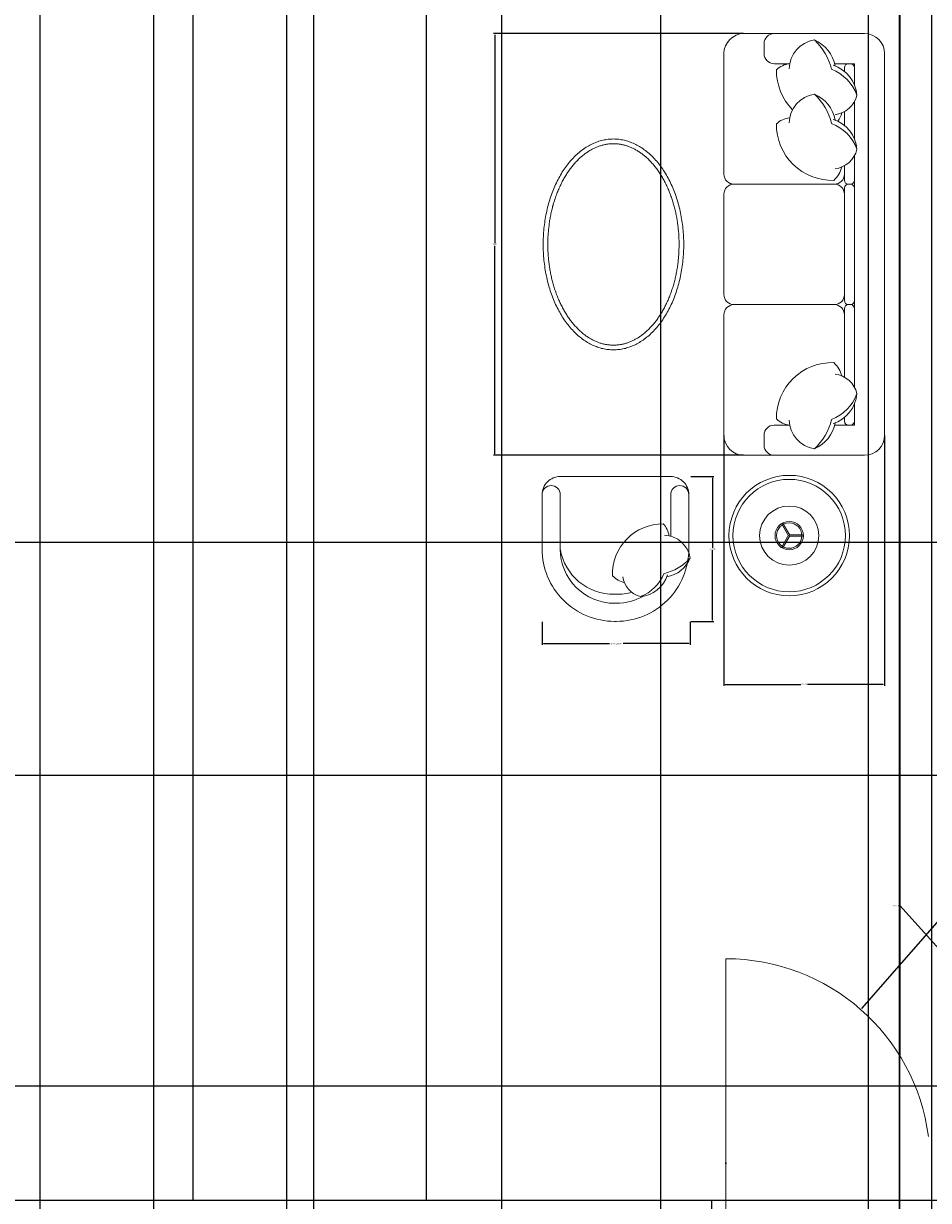
# Model space of a CAD drawing. Units: inches. Extents: x 1861 to 2564, y 1482 to 2317.
# Tile 5 of 11: x 2090 to 2217, y 1853 to 2018. Entities that reach past the tile are written whole.
import ezdxf

# ---------------------------------------------------------------- set-up
doc = ezdxf.new("R2010")
doc.units = ezdxf.units.IN
for name, color, linetype, lineweight in [('A-ANNO-DIMS', 2, 'Continuous', 18), ('A-DOOR', 3, 'Continuous', 18), ('A-FURN', 8, 'Continuous', 13), ('A-WALL', 7, 'Continuous', 35)]:
    doc.layers.add(name, color=color, linetype=linetype, lineweight=lineweight)
doc.styles.get("Standard").update_dxf_attribs({"font": 'arial.ttf'})
doc.dimstyles.get("Standard").update_dxf_attribs({"dimtxt": 0.18, "dimasz": 0.18, "dimexe": 0.18, "dimexo": 0.0625, "dimgap": 0.09, "dimtad": 0, "dimtih": 1, "dimtoh": 1, "dimdec": 4, "dimzin": 0, "dimdsep": 46, "dimtxsty": 'Standard', "dimcen": 0.09, "dimadec": 0, "dimazin": 0, "dimtfac": 1, "dimtdec": 4, "dimtofl": 0, "dimtmove": 0, "dimatfit": 3, "dimfxl": 1, "dimtolj": 1, "dimtzin": 0, "dimarcsym": 0})

# ---------------------------------------------------------------- blocks, each defined once
blk = doc.blocks.new('TABLE-SIDE-ROUND')
at = {"ltscale": 0.03}
for p, q in [((8.34, 8.45), (9.33, 10.16)), ((8.49, 8.36), (9.48, 10.08)), ((8.41, 8.5), (6.44, 8.5)), ((8.41, 8.32), (6.44, 8.32)), ((8.34, 8.36), (9.33, 6.65)), ((8.49, 8.45), (9.48, 6.74))]:
    blk.add_line(p, q, dxfattribs=at)
for radius in [8.41, 4.13, 1.98, 1.77]:
    blk.add_circle((8.41, 8.41), radius, dxfattribs=at)
blk.add_circle((8.41, 8.41), 7.85)
blk = doc.blocks.new('CHAIR-LOUNGE')
at = {"ltscale": 0.03}
blk.add_lwpolyline([(10.44, 0), (18.15, 0, 0.414214), (20.68, 2.53), (20.68, 10.11, 0.414214), (10.57, 20.22), (10.44, 20.22), (10.32, 20.22, 0.414214), (0.21, 10.11), (0.21, 2.53, 0.414214), (2.73, 0), (10.44, 0)], format="xyb", dxfattribs=at)
for points in [[(0, 11.38, -0.14773), (3.69, 13.56, -0.213343), (6.95, 16.74, -0.178662)], [(3.18, 13.73, -0.306663), (6.95, 16.74, -0.30633), (9.42, 13.99, 0.872847)], [(6.55, 16.69, -0.130591), (10.32, 17.69), (10.44, 17.69)], [(18.15, 10.11, 0.414214), (10.57, 17.69), (10.44, 17.69)], [(2.98, 8.28, 0.165541), (3.77, 6.61, 0.425989), (10.86, 13.85, 0.121523), (9.18, 14.84, -7.115464)], [(8.16, 16.16, -0.072384), (10.32, 16.43), (10.44, 16.43)], [(18.15, 10.11, 0.372719), (10.57, 16.43), (10.44, 16.43)], [(3.62, 8.2, -0.356772), (0, 11.38, -0.249542), (3.28, 14.01, 9.61688)], [(18.15, 10.11), (18.15, 2.53, 0.414214), (19.42, 1.26), (19.42, 1.26, 0.414214), (20.68, 2.53)], [(2.73, 8.34), (2.73, 2.53, -0.414214), (1.47, 1.26), (1.47, 1.26, -0.414214), (0.21, 2.53)]]:
    blk.add_lwpolyline(points, format="xyb")
blk = doc.blocks.new('TABLE-COFFEE-OVAL')
at = {"ltscale": 0.03}
blk.add_polyline3d([(9.81, 29.44, 0), (9.63, 29.44, 0), (9.44, 29.43, 0), (9.26, 29.41, 0), (9.07, 29.4, 0), (8.89, 29.37, 0), (8.7, 29.34, 0), (8.52, 29.31, 0), (8.33, 29.27, 0), (8.15, 29.23, 0), (7.97, 29.18, 0), (7.79, 29.12, 0), (7.6, 29.06, 0), (7.42, 28.99, 0), (7.24, 28.92, 0), (7.07, 28.85, 0), (6.89, 28.77, 0), (6.71, 28.68, 0), (6.54, 28.59, 0), (6.36, 28.5, 0), (6.19, 28.4, 0), (6.02, 28.29, 0), (5.85, 28.18, 0), (5.68, 28.07, 0), (5.51, 27.95, 0), (5.34, 27.82, 0), (5.18, 27.69, 0), (5.02, 27.56, 0), (4.85, 27.42, 0), (4.69, 27.28, 0), (4.54, 27.13, 0), (4.38, 26.98, 0), (4.23, 26.82, 0), (4.08, 26.66, 0), (3.93, 26.49, 0), (3.78, 26.33, 0), (3.63, 26.15, 0), (3.49, 25.97, 0), (3.35, 25.79, 0), (3.21, 25.61, 0), (3.08, 25.42, 0), (2.94, 25.23, 0), (2.81, 25.03, 0), (2.68, 24.83, 0), (2.56, 24.62, 0), (2.43, 24.42, 0), (2.31, 24.2, 0), (2.19, 23.99, 0), (2.08, 23.77, 0), (1.96, 23.55, 0), (1.85, 23.33, 0), (1.75, 23.1, 0), (1.64, 22.87, 0), (1.54, 22.63, 0), (1.44, 22.4, 0), (1.35, 22.16, 0), (1.26, 21.92, 0), (1.17, 21.67, 0), (1.08, 21.43, 0), (1, 21.18, 0), (0.92, 20.93, 0), (0.84, 20.67, 0), (0.77, 20.42, 0), (0.7, 20.16, 0), (0.63, 19.9, 0), (0.57, 19.64, 0), (0.51, 19.37, 0), (0.45, 19.11, 0), (0.39, 18.84, 0), (0.34, 18.57, 0), (0.3, 18.31, 0), (0.25, 18.03, 0), (0.21, 17.76, 0), (0.18, 17.49, 0), (0.14, 17.22, 0), (0.11, 16.94, 0), (0.09, 16.66, 0), (0.07, 16.39, 0), (0.05, 16.11, 0), (0.03, 15.83, 0), (0.02, 15.56, 0), (0.01, 15.28, 0), (0, 15, 0), (0, 14.72, 0), (0, 14.44, 0), (0.01, 14.16, 0), (0.02, 13.89, 0), (0.03, 13.61, 0), (0.05, 13.33, 0), (0.07, 13.05, 0), (0.09, 12.78, 0), (0.11, 12.5, 0), (0.14, 12.23, 0), (0.18, 11.95, 0), (0.21, 11.68, 0), (0.25, 11.41, 0), (0.3, 11.14, 0), (0.34, 10.87, 0), (0.39, 10.6, 0), (0.45, 10.33, 0), (0.51, 10.07, 0), (0.57, 9.8, 0), (0.63, 9.54, 0), (0.7, 9.28, 0), (0.77, 9.02, 0), (0.84, 8.77, 0), (0.92, 8.52, 0), (1, 8.26, 0), (1.08, 8.01, 0), (1.17, 7.77, 0), (1.26, 7.52, 0), (1.35, 7.28, 0), (1.44, 7.04, 0), (1.54, 6.81, 0), (1.64, 6.57, 0), (1.75, 6.34, 0), (1.85, 6.12, 0), (1.96, 5.89, 0), (2.08, 5.67, 0), (2.19, 5.45, 0), (2.31, 5.24, 0), (2.43, 5.03, 0), (2.56, 4.82, 0), (2.68, 4.61, 0), (2.81, 4.41, 0), (2.94, 4.22, 0), (3.08, 4.02, 0), (3.21, 3.83, 0), (3.35, 3.65, 0), (3.49, 3.47, 0), (3.63, 3.29, 0), (3.78, 3.12, 0), (3.93, 2.95, 0), (4.08, 2.78, 0), (4.23, 2.62, 0), (4.38, 2.46, 0), (4.54, 2.31, 0), (4.69, 2.17, 0), (4.85, 2.02, 0), (5.02, 1.88, 0), (5.18, 1.75, 0), (5.34, 1.62, 0), (5.51, 1.5, 0), (5.68, 1.38, 0), (5.85, 1.26, 0), (6.02, 1.15, 0), (6.19, 1.05, 0), (6.36, 0.94, 0), (6.54, 0.85, 0), (6.71, 0.76, 0), (6.89, 0.67, 0), (7.07, 0.59, 0), (7.24, 0.52, 0), (7.42, 0.45, 0), (7.6, 0.38, 0), (7.79, 0.32, 0), (7.97, 0.27, 0), (8.15, 0.22, 0), (8.33, 0.17, 0), (8.52, 0.13, 0), (8.7, 0.1, 0), (8.89, 0.07, 0), (9.07, 0.05, 0), (9.26, 0.03, 0), (9.44, 0.01, 0), (9.63, 0.01, 0), (9.81, 0, 0), (10, 0.01, 0), (10.18, 0.01, 0), (10.37, 0.03, 0), (10.56, 0.05, 0), (10.74, 0.07, 0), (10.93, 0.1, 0), (11.11, 0.13, 0), (11.29, 0.17, 0), (11.48, 0.22, 0), (11.66, 0.27, 0), (11.84, 0.32, 0), (12.02, 0.38, 0), (12.2, 0.45, 0), (12.38, 0.52, 0), (12.56, 0.59, 0), (12.74, 0.67, 0), (12.92, 0.76, 0), (13.09, 0.85, 0), (13.27, 0.94, 0), (13.44, 1.05, 0), (13.61, 1.15, 0), (13.78, 1.26, 0), (13.95, 1.38, 0), (14.12, 1.5, 0), (14.28, 1.62, 0), (14.45, 1.75, 0), (14.61, 1.88, 0), (14.77, 2.02, 0), (14.93, 2.17, 0), (15.09, 2.31, 0), (15.25, 2.46, 0), (15.4, 2.62, 0), (15.55, 2.78, 0), (15.7, 2.95, 0), (15.85, 3.12, 0), (15.99, 3.29, 0), (16.14, 3.47, 0), (16.28, 3.65, 0), (16.42, 3.83, 0), (16.55, 4.02, 0), (16.69, 4.22, 0), (16.82, 4.41, 0), (16.95, 4.61, 0), (17.07, 4.82, 0), (17.2, 5.03, 0), (17.32, 5.24, 0), (17.43, 5.45, 0), (17.55, 5.67, 0), (17.66, 5.89, 0), (17.77, 6.12, 0), (17.88, 6.34, 0), (17.98, 6.57, 0), (18.09, 6.81, 0), (18.18, 7.04, 0), (18.28, 7.28, 0), (18.37, 7.52, 0), (18.46, 7.77, 0), (18.55, 8.01, 0), (18.63, 8.26, 0), (18.71, 8.52, 0), (18.79, 8.77, 0), (18.86, 9.02, 0), (18.93, 9.28, 0), (19, 9.54, 0), (19.06, 9.8, 0), (19.12, 10.07, 0), (19.18, 10.33, 0), (19.23, 10.6, 0), (19.28, 10.87, 0), (19.33, 11.14, 0), (19.37, 11.41, 0), (19.41, 11.68, 0), (19.45, 11.95, 0), (19.48, 12.23, 0), (19.51, 12.5, 0), (19.54, 12.78, 0), (19.56, 13.05, 0), (19.58, 13.33, 0), (19.6, 13.61, 0), (19.61, 13.89, 0), (19.62, 14.16, 0), (19.62, 14.44, 0), (19.63, 14.72, 0), (19.62, 15, 0), (19.62, 15.28, 0), (19.61, 15.56, 0), (19.6, 15.83, 0), (19.58, 16.11, 0), (19.56, 16.39, 0), (19.54, 16.66, 0), (19.51, 16.94, 0), (19.48, 17.22, 0), (19.45, 17.49, 0), (19.41, 17.76, 0), (19.37, 18.03, 0), (19.33, 18.31, 0), (19.28, 18.57, 0), (19.23, 18.84, 0), (19.18, 19.11, 0), (19.12, 19.37, 0), (19.06, 19.64, 0), (19, 19.9, 0), (18.93, 20.16, 0), (18.86, 20.42, 0), (18.79, 20.67, 0), (18.71, 20.93, 0), (18.63, 21.18, 0), (18.55, 21.43, 0), (18.46, 21.67, 0), (18.37, 21.92, 0), (18.28, 22.16, 0), (18.18, 22.4, 0), (18.09, 22.63, 0), (17.98, 22.87, 0), (17.88, 23.1, 0), (17.77, 23.33, 0), (17.66, 23.55, 0), (17.55, 23.77, 0), (17.43, 23.99, 0), (17.32, 24.2, 0), (17.2, 24.42, 0), (17.07, 24.62, 0), (16.95, 24.83, 0), (16.82, 25.03, 0), (16.69, 25.23, 0), (16.55, 25.42, 0), (16.42, 25.61, 0), (16.28, 25.79, 0), (16.14, 25.97, 0), (15.99, 26.15, 0), (15.85, 26.33, 0), (15.7, 26.49, 0), (15.55, 26.66, 0), (15.4, 26.82, 0), (15.25, 26.98, 0), (15.09, 27.13, 0), (14.93, 27.28, 0), (14.77, 27.42, 0), (14.61, 27.56, 0), (14.45, 27.69, 0), (14.28, 27.82, 0), (14.12, 27.95, 0), (13.95, 28.07, 0), (13.78, 28.18, 0), (13.61, 28.29, 0), (13.44, 28.4, 0), (13.27, 28.5, 0), (13.09, 28.59, 0), (12.92, 28.68, 0), (12.74, 28.77, 0), (12.56, 28.85, 0), (12.38, 28.92, 0), (12.2, 28.99, 0), (12.02, 29.06, 0), (11.84, 29.12, 0), (11.66, 29.18, 0), (11.48, 29.23, 0), (11.29, 29.27, 0), (11.11, 29.31, 0), (10.93, 29.34, 0), (10.74, 29.37, 0), (10.56, 29.4, 0), (10.37, 29.41, 0), (10.18, 29.43, 0), (10, 29.44, 0), (9.81, 29.44, 0)], dxfattribs=at)
blk.add_polyline3d([(9.81, 28.78, 0), (9.71, 28.78, 0), (9.61, 28.78, 0), (9.51, 28.78, 0), (9.41, 28.77, 0), (9.31, 28.76, 0), (9.2, 28.75, 0), (9.1, 28.74, 0), (9, 28.73, 0), (8.89, 28.71, 0), (8.79, 28.69, 0), (8.69, 28.68, 0), (8.58, 28.65, 0), (8.48, 28.63, 0), (8.37, 28.61, 0), (8.27, 28.58, 0), (8.16, 28.55, 0), (8.05, 28.52, 0), (7.95, 28.49, 0), (7.84, 28.45, 0), (7.73, 28.41, 0), (7.63, 28.37, 0), (7.52, 28.33, 0), (7.41, 28.29, 0), (7.31, 28.24, 0), (7.2, 28.19, 0), (7.09, 28.14, 0), (6.98, 28.09, 0), (6.88, 28.03, 0), (6.77, 27.97, 0), (6.66, 27.91, 0), (6.55, 27.85, 0), (6.45, 27.79, 0), (6.34, 27.72, 0), (6.23, 27.65, 0), (6.13, 27.58, 0), (6.02, 27.51, 0), (5.92, 27.43, 0), (5.81, 27.36, 0), (5.71, 27.28, 0), (5.6, 27.19, 0), (5.5, 27.11, 0), (5.39, 27.02, 0), (5.29, 26.93, 0), (5.19, 26.84, 0), (5.09, 26.75, 0), (4.98, 26.65, 0), (4.88, 26.55, 0), (4.78, 26.45, 0), (4.68, 26.34, 0), (4.58, 26.24, 0), (4.49, 26.13, 0), (4.39, 26.02, 0), (4.29, 25.91, 0), (4.2, 25.79, 0), (4.1, 25.68, 0), (4.01, 25.56, 0), (3.91, 25.44, 0), (3.82, 25.32, 0), (3.73, 25.19, 0), (3.64, 25.07, 0), (3.55, 24.94, 0), (3.46, 24.81, 0), (3.37, 24.68, 0), (3.29, 24.54, 0), (3.2, 24.41, 0), (3.12, 24.27, 0), (3.03, 24.13, 0), (2.95, 23.99, 0), (2.87, 23.85, 0), (2.79, 23.71, 0), (2.71, 23.56, 0), (2.63, 23.41, 0), (2.56, 23.27, 0), (2.48, 23.12, 0), (2.41, 22.97, 0), (2.34, 22.81, 0), (2.27, 22.66, 0), (2.2, 22.51, 0), (2.13, 22.35, 0), (2.07, 22.19, 0), (2, 22.04, 0), (1.94, 21.88, 0), (1.88, 21.72, 0), (1.82, 21.55, 0), (1.76, 21.39, 0), (1.7, 21.23, 0), (1.65, 21.07, 0), (1.6, 20.9, 0), (1.54, 20.74, 0), (1.49, 20.58, 0), (1.44, 20.41, 0), (1.4, 20.25, 0), (1.35, 20.08, 0), (1.31, 19.92, 0), (1.26, 19.75, 0), (1.22, 19.59, 0), (1.18, 19.42, 0), (1.15, 19.25, 0), (1.11, 19.09, 0), (1.07, 18.92, 0), (1.04, 18.75, 0), (1.01, 18.58, 0), (0.98, 18.42, 0), (0.95, 18.25, 0), (0.92, 18.08, 0), (0.89, 17.91, 0), (0.87, 17.74, 0), (0.84, 17.57, 0), (0.82, 17.4, 0), (0.8, 17.23, 0), (0.78, 17.06, 0), (0.76, 16.89, 0), (0.75, 16.72, 0), (0.73, 16.55, 0), (0.72, 16.38, 0), (0.71, 16.21, 0), (0.7, 16.04, 0), (0.69, 15.87, 0), (0.68, 15.7, 0), (0.67, 15.53, 0), (0.67, 15.36, 0), (0.66, 15.19, 0), (0.66, 15.02, 0), (0.66, 14.85, 0), (0.66, 14.68, 0), (0.66, 14.51, 0), (0.66, 14.34, 0), (0.66, 14.17, 0), (0.67, 14, 0), (0.67, 13.82, 0), (0.68, 13.65, 0), (0.69, 13.48, 0), (0.7, 13.31, 0), (0.71, 13.14, 0), (0.73, 12.97, 0), (0.74, 12.8, 0), (0.76, 12.63, 0), (0.77, 12.46, 0), (0.79, 12.29, 0), (0.81, 12.12, 0), (0.83, 11.95, 0), (0.86, 11.78, 0), (0.88, 11.62, 0), (0.91, 11.45, 0), (0.93, 11.28, 0), (0.96, 11.11, 0), (0.99, 10.94, 0), (1.02, 10.77, 0), (1.06, 10.61, 0), (1.09, 10.44, 0), (1.13, 10.27, 0), (1.16, 10.1, 0), (1.2, 9.94, 0), (1.24, 9.77, 0), (1.29, 9.61, 0), (1.33, 9.44, 0), (1.37, 9.28, 0), (1.42, 9.11, 0), (1.47, 8.95, 0), (1.52, 8.78, 0), (1.57, 8.62, 0), (1.62, 8.46, 0), (1.68, 8.29, 0), (1.73, 8.13, 0), (1.79, 7.97, 0), (1.85, 7.81, 0), (1.91, 7.65, 0), (1.97, 7.49, 0), (2.03, 7.33, 0), (2.1, 7.17, 0), (2.17, 7.01, 0), (2.23, 6.86, 0), (2.3, 6.7, 0), (2.37, 6.55, 0), (2.45, 6.4, 0), (2.52, 6.25, 0), (2.6, 6.1, 0), (2.67, 5.95, 0), (2.75, 5.81, 0), (2.83, 5.66, 0), (2.91, 5.52, 0), (2.99, 5.38, 0), (3.07, 5.24, 0), (3.16, 5.1, 0), (3.24, 4.97, 0), (3.33, 4.83, 0), (3.42, 4.7, 0), (3.5, 4.57, 0), (3.59, 4.44, 0), (3.68, 4.31, 0), (3.77, 4.19, 0), (3.87, 4.06, 0), (3.96, 3.94, 0), (4.05, 3.82, 0), (4.15, 3.71, 0), (4.24, 3.59, 0), (4.34, 3.48, 0), (4.44, 3.37, 0), (4.53, 3.26, 0), (4.63, 3.15, 0), (4.73, 3.04, 0), (4.83, 2.94, 0), (4.93, 2.84, 0), (5.03, 2.74, 0), (5.14, 2.65, 0), (5.24, 2.56, 0), (5.34, 2.47, 0), (5.44, 2.38, 0), (5.55, 2.29, 0), (5.65, 2.21, 0), (5.76, 2.13, 0), (5.86, 2.05, 0), (5.97, 1.97, 0), (6.07, 1.9, 0), (6.18, 1.82, 0), (6.29, 1.75, 0), (6.39, 1.69, 0), (6.5, 1.62, 0), (6.61, 1.56, 0), (6.72, 1.5, 0), (6.82, 1.44, 0), (6.93, 1.38, 0), (7.04, 1.33, 0), (7.14, 1.28, 0), (7.25, 1.23, 0), (7.36, 1.18, 0), (7.47, 1.13, 0), (7.57, 1.09, 0), (7.68, 1.05, 0), (7.79, 1.01, 0), (7.89, 0.97, 0), (8, 0.94, 0), (8.11, 0.91, 0), (8.21, 0.88, 0), (8.32, 0.85, 0), (8.42, 0.82, 0), (8.53, 0.8, 0), (8.63, 0.78, 0), (8.74, 0.76, 0), (8.84, 0.74, 0), (8.95, 0.72, 0), (9.05, 0.71, 0), (9.15, 0.69, 0), (9.26, 0.68, 0), (9.36, 0.68, 0), (9.46, 0.67, 0), (9.56, 0.66, 0), (9.66, 0.66, 0), (9.76, 0.66, 0), (9.86, 0.66, 0), (9.96, 0.66, 0), (10.07, 0.66, 0), (10.17, 0.67, 0), (10.27, 0.68, 0), (10.37, 0.68, 0), (10.47, 0.69, 0), (10.58, 0.71, 0), (10.68, 0.72, 0), (10.78, 0.74, 0), (10.89, 0.76, 0), (10.99, 0.78, 0), (11.1, 0.8, 0), (11.2, 0.82, 0), (11.31, 0.85, 0), (11.41, 0.88, 0), (11.52, 0.91, 0), (11.63, 0.94, 0), (11.73, 0.97, 0), (11.84, 1.01, 0), (11.95, 1.05, 0), (12.05, 1.09, 0), (12.16, 1.13, 0), (12.27, 1.18, 0), (12.37, 1.23, 0), (12.48, 1.28, 0), (12.59, 1.33, 0), (12.7, 1.38, 0), (12.8, 1.44, 0), (12.91, 1.5, 0), (13.02, 1.56, 0), (13.13, 1.62, 0), (13.23, 1.69, 0), (13.34, 1.75, 0), (13.45, 1.82, 0), (13.55, 1.9, 0), (13.66, 1.97, 0), (13.76, 2.05, 0), (13.87, 2.13, 0), (13.97, 2.21, 0), (14.08, 2.29, 0), (14.18, 2.38, 0), (14.29, 2.47, 0), (14.39, 2.56, 0), (14.49, 2.65, 0), (14.59, 2.74, 0), (14.69, 2.84, 0), (14.79, 2.94, 0), (14.89, 3.04, 0), (14.99, 3.15, 0), (15.09, 3.26, 0), (15.19, 3.37, 0), (15.29, 3.48, 0), (15.38, 3.59, 0), (15.48, 3.71, 0), (15.57, 3.82, 0), (15.67, 3.94, 0), (15.76, 4.06, 0), (15.85, 4.19, 0), (15.94, 4.31, 0), (16.03, 4.44, 0), (16.12, 4.57, 0), (16.21, 4.7, 0), (16.3, 4.83, 0), (16.38, 4.97, 0), (16.47, 5.1, 0), (16.55, 5.24, 0), (16.64, 5.38, 0), (16.72, 5.52, 0), (16.8, 5.66, 0), (16.88, 5.81, 0), (16.95, 5.95, 0), (17.03, 6.1, 0), (17.11, 6.25, 0), (17.18, 6.4, 0), (17.25, 6.55, 0), (17.32, 6.7, 0), (17.39, 6.86, 0), (17.46, 7.01, 0), (17.53, 7.17, 0), (17.59, 7.33, 0), (17.66, 7.49, 0), (17.72, 7.65, 0), (17.78, 7.81, 0), (17.84, 7.97, 0), (17.9, 8.13, 0), (17.95, 8.29, 0), (18.01, 8.46, 0), (18.06, 8.62, 0), (18.11, 8.78, 0), (18.16, 8.95, 0), (18.21, 9.11, 0), (18.25, 9.28, 0), (18.3, 9.44, 0), (18.34, 9.61, 0), (18.38, 9.77, 0), (18.42, 9.94, 0), (18.46, 10.1, 0), (18.5, 10.27, 0), (18.54, 10.44, 0), (18.57, 10.61, 0), (18.6, 10.77, 0), (18.63, 10.94, 0), (18.66, 11.11, 0), (18.69, 11.28, 0), (18.72, 11.45, 0), (18.75, 11.62, 0), (18.77, 11.78, 0), (18.79, 11.95, 0), (18.81, 12.12, 0), (18.83, 12.29, 0), (18.85, 12.46, 0), (18.87, 12.63, 0), (18.89, 12.8, 0), (18.9, 12.97, 0), (18.91, 13.14, 0), (18.93, 13.31, 0), (18.94, 13.48, 0), (18.95, 13.65, 0), (18.95, 13.82, 0), (18.96, 14, 0), (18.96, 14.17, 0), (18.97, 14.34, 0), (18.97, 14.51, 0), (18.97, 14.68, 0), (18.97, 14.85, 0), (18.97, 15.02, 0), (18.97, 15.19, 0), (18.96, 15.36, 0), (18.96, 15.53, 0), (18.95, 15.7, 0), (18.94, 15.87, 0), (18.93, 16.04, 0), (18.92, 16.21, 0), (18.91, 16.38, 0), (18.89, 16.55, 0), (18.88, 16.72, 0), (18.86, 16.89, 0), (18.84, 17.06, 0), (18.83, 17.23, 0), (18.8, 17.4, 0), (18.78, 17.57, 0), (18.76, 17.74, 0), (18.73, 17.91, 0), (18.71, 18.08, 0), (18.68, 18.25, 0), (18.65, 18.42, 0), (18.62, 18.58, 0), (18.59, 18.75, 0), (18.55, 18.92, 0), (18.52, 19.09, 0), (18.48, 19.25, 0), (18.44, 19.42, 0), (18.4, 19.59, 0), (18.36, 19.75, 0), (18.32, 19.92, 0), (18.28, 20.08, 0), (18.23, 20.25, 0), (18.18, 20.41, 0), (18.13, 20.58, 0), (18.08, 20.74, 0), (18.03, 20.9, 0), (17.98, 21.07, 0), (17.92, 21.23, 0), (17.87, 21.39, 0), (17.81, 21.55, 0), (17.75, 21.72, 0), (17.69, 21.88, 0), (17.62, 22.04, 0), (17.56, 22.19, 0), (17.49, 22.35, 0), (17.43, 22.51, 0), (17.36, 22.66, 0), (17.29, 22.81, 0), (17.22, 22.97, 0), (17.14, 23.12, 0), (17.07, 23.27, 0), (16.99, 23.41, 0), (16.92, 23.56, 0), (16.84, 23.71, 0), (16.76, 23.85, 0), (16.68, 23.99, 0), (16.59, 24.13, 0), (16.51, 24.27, 0), (16.43, 24.41, 0), (16.34, 24.54, 0), (16.26, 24.68, 0), (16.17, 24.81, 0), (16.08, 24.94, 0), (15.99, 25.07, 0), (15.9, 25.19, 0), (15.81, 25.32, 0), (15.71, 25.44, 0), (15.62, 25.56, 0), (15.53, 25.68, 0), (15.43, 25.79, 0), (15.34, 25.91, 0), (15.24, 26.02, 0), (15.14, 26.13, 0), (15.04, 26.24, 0), (14.94, 26.34, 0), (14.84, 26.45, 0), (14.74, 26.55, 0), (14.64, 26.65, 0), (14.54, 26.75, 0), (14.44, 26.84, 0), (14.34, 26.93, 0), (14.23, 27.02, 0), (14.13, 27.11, 0), (14.03, 27.19, 0), (13.92, 27.28, 0), (13.82, 27.36, 0), (13.71, 27.43, 0), (13.61, 27.51, 0), (13.5, 27.58, 0), (13.39, 27.65, 0), (13.29, 27.72, 0), (13.18, 27.79, 0), (13.07, 27.85, 0), (12.97, 27.91, 0), (12.86, 27.97, 0), (12.75, 28.03, 0), (12.64, 28.09, 0), (12.54, 28.14, 0), (12.43, 28.19, 0), (12.32, 28.24, 0), (12.21, 28.29, 0), (12.11, 28.33, 0), (12, 28.37, 0), (11.89, 28.41, 0), (11.79, 28.45, 0), (11.68, 28.49, 0), (11.57, 28.52, 0), (11.47, 28.55, 0), (11.36, 28.58, 0), (11.26, 28.61, 0), (11.15, 28.63, 0), (11.05, 28.65, 0), (10.94, 28.68, 0), (10.84, 28.69, 0), (10.73, 28.71, 0), (10.63, 28.73, 0), (10.53, 28.74, 0), (10.42, 28.75, 0), (10.32, 28.76, 0), (10.22, 28.77, 0), (10.12, 28.78, 0), (10.01, 28.78, 0), (9.91, 28.78, 0), (9.81, 28.78, 0)])
blk = doc.blocks.new('*D26')
at = {"layer": 'A-ANNO-DIMS', "color": 0, "lineweight": -2, "transparency": 16777216}
for p, q in [((2162.87, 1934.17), (2162.87, 1930.95)), ((2183.55, 1934.17), (2183.55, 1930.95)), ((2163.05, 1931.13), (2172.26, 1931.13)), ((2183.37, 1931.13), (2174.17, 1931.13))]:
    blk.add_line(p, q, dxfattribs=at)
at = {"layer": 'A-ANNO-DIMS', "color": 0, "transparency": 16777216}
for points in [[(2163.05, 1931.16), (2163.05, 1931.1), (2162.87, 1931.13)], [(2183.37, 1931.16), (2183.37, 1931.1), (2183.55, 1931.13)]]:
    blk.add_solid(points, dxfattribs=at)
at = {"layer": 'Defpoints', "color": 0, "transparency": 16777216}
for p in [(2162.87, 1934.23), (2183.55, 1934.23), (2162.87, 1931.13)]:
    blk.add_point(p, dxfattribs=at)
at = {"layer": 'A-ANNO-DIMS', "color": 0, "transparency": 16777216, "insert": (2173.21, 1931.13), "char_height": 0.18, "attachment_point": 5}
blk.add_mtext('\\A1;CHAIR 21 TYP.', dxfattribs=at)
blk = doc.blocks.new('*D27')
at = {"layer": 'A-ANNO-DIMS', "color": 0, "lineweight": -2, "transparency": 16777216}
for p, q in [((2183.62, 1954.45), (2186.84, 1954.45)), ((2186.66, 1954.27), (2186.66, 1944.52)), ((2186.66, 1934.41), (2186.66, 1944.16)), ((2183.62, 1934.23), (2186.84, 1934.23))]:
    blk.add_line(p, q, dxfattribs=at)
at = {"layer": 'A-ANNO-DIMS', "color": 0, "transparency": 16777216}
for points in [[(2186.63, 1954.27), (2186.69, 1954.27), (2186.66, 1954.45)], [(2186.63, 1934.41), (2186.69, 1934.41), (2186.66, 1934.23)]]:
    blk.add_solid(points, dxfattribs=at)
at = {"layer": 'Defpoints', "color": 0, "transparency": 16777216}
for p in [(2183.55, 1954.45), (2183.55, 1934.23), (2186.66, 1934.23)]:
    blk.add_point(p, dxfattribs=at)
at = {"layer": 'A-ANNO-DIMS', "color": 0, "transparency": 16777216, "insert": (2186.66, 1944.34), "char_height": 0.18, "attachment_point": 5}
blk.add_mtext('\\A1;20 TYP.', dxfattribs=at)
blk = doc.blocks.new('*D36')
at = {"layer": 'A-ANNO-DIMS', "color": 0, "lineweight": -2, "transparency": 16777216}
for p, q in [((2092.74, 2250.82), (2092.74, 1545.6)), ((2127.18, 2250.82), (2127.18, 1545.6)), ((2092.92, 1545.78), (2109.5, 1545.78)), ((2127, 1545.78), (2110.43, 1545.78))]:
    blk.add_line(p, q, dxfattribs=at)
at = {"layer": 'A-ANNO-DIMS', "color": 0, "transparency": 16777216}
for points in [[(2092.92, 1545.81), (2092.92, 1545.75), (2092.74, 1545.78)], [(2127, 1545.81), (2127, 1545.75), (2127.18, 1545.78)]]:
    blk.add_solid(points, dxfattribs=at)
at = {"layer": 'Defpoints', "color": 0, "transparency": 16777216}
for p in [(2092.74, 2250.89), (2127.18, 2250.89), (2127.18, 1545.78)]:
    blk.add_point(p, dxfattribs=at)
at = {"layer": 'A-ANNO-DIMS', "color": 0, "transparency": 16777216, "insert": (2109.96, 1545.78), "char_height": 0.18, "attachment_point": 5}
blk.add_mtext('\\A1;34.445', dxfattribs=at)
blk = doc.blocks.new('*D52')
at = {"layer": 'A-ANNO-DIMS', "color": 0, "lineweight": -2, "transparency": 16777216}
for p, q in [((2179.39, 2154.82), (2179.39, 1545.6)), ((2208.37, 2154.82), (2208.37, 1545.6)), ((2179.57, 1545.78), (2193.49, 1545.78)), ((2208.19, 1545.78), (2194.28, 1545.78))]:
    blk.add_line(p, q, dxfattribs=at)
at = {"layer": 'A-ANNO-DIMS', "color": 0, "transparency": 16777216}
for points in [[(2179.57, 1545.81), (2179.57, 1545.75), (2179.39, 1545.78)], [(2208.19, 1545.81), (2208.19, 1545.75), (2208.37, 1545.78)]]:
    blk.add_solid(points, dxfattribs=at)
at = {"layer": 'Defpoints', "color": 0, "transparency": 16777216}
for p in [(2179.39, 2154.89), (2208.37, 2154.89), (2208.37, 1545.78)]:
    blk.add_point(p, dxfattribs=at)
at = {"layer": 'A-ANNO-DIMS', "color": 0, "transparency": 16777216, "insert": (2193.88, 1545.78), "char_height": 0.18, "attachment_point": 5}
blk.add_mtext('\\A1;28.98', dxfattribs=at)
blk = doc.blocks.new('*D53')
at = {"layer": 'A-ANNO-DIMS', "color": 0, "lineweight": -2, "transparency": 16777216}
for p, q in [((2076.3, 1945.29), (2537.22, 1945.29)), ((2537.04, 1945.11), (2537.04, 1929.2)), ((2537.04, 1912.93), (2537.04, 1928.84)), ((2076.3, 1912.75), (2537.22, 1912.75))]:
    blk.add_line(p, q, dxfattribs=at)
at = {"layer": 'A-ANNO-DIMS', "color": 0, "transparency": 16777216}
for points in [[(2537.01, 1945.11), (2537.07, 1945.11), (2537.04, 1945.29)], [(2537.01, 1912.93), (2537.07, 1912.93), (2537.04, 1912.75)]]:
    blk.add_solid(points, dxfattribs=at)
at = {"layer": 'Defpoints', "color": 0, "transparency": 16777216}
for p in [(2076.24, 1945.29), (2537.04, 1945.29), (2076.24, 1912.75)]:
    blk.add_point(p, dxfattribs=at)
at = {"layer": 'A-ANNO-DIMS', "color": 0, "transparency": 16777216, "insert": (2537.04, 1929.02), "char_height": 0.18, "attachment_point": 5}
blk.add_mtext('\\A1;32.544', dxfattribs=at)
blk = doc.blocks.new('*D55')
at = {"layer": 'A-ANNO-DIMS', "color": 0, "lineweight": -2, "transparency": 16777216}
for p, q in [((2114.18, 1853.45), (2114.18, 2290.37)), ((2114.36, 2290.19), (2130, 2290.19)), ((2146.56, 2290.19), (2130.92, 2290.19)), ((2146.74, 1853.45), (2146.74, 2290.37))]:
    blk.add_line(p, q, dxfattribs=at)
at = {"layer": 'A-ANNO-DIMS', "color": 0, "transparency": 16777216}
for points in [[(2114.36, 2290.22), (2114.36, 2290.16), (2114.18, 2290.19)], [(2146.56, 2290.22), (2146.56, 2290.16), (2146.74, 2290.19)]]:
    blk.add_solid(points, dxfattribs=at)
at = {"layer": 'Defpoints', "color": 0, "transparency": 16777216}
for p in [(2146.74, 2290.19), (2114.18, 1853.39), (2146.74, 1853.39)]:
    blk.add_point(p, dxfattribs=at)
at = {"layer": 'A-ANNO-DIMS', "color": 0, "transparency": 16777216, "insert": (2130.46, 2290.19), "char_height": 0.18, "attachment_point": 5}
blk.add_mtext('\\A1;32.564', dxfattribs=at)
blk = doc.blocks.new('*D56')
at = {"layer": 'A-ANNO-DIMS', "color": 0, "lineweight": -2, "transparency": 16777216}
for p, q in [((2186.51, 1853.32), (2186.51, 1545.6)), ((2244.44, 1853.32), (2244.44, 1545.6)), ((2186.69, 1545.78), (2215.08, 1545.78)), ((2244.26, 1545.78), (2215.87, 1545.78))]:
    blk.add_line(p, q, dxfattribs=at)
at = {"layer": 'A-ANNO-DIMS', "color": 0, "transparency": 16777216}
for points in [[(2186.69, 1545.81), (2186.69, 1545.75), (2186.51, 1545.78)], [(2244.26, 1545.81), (2244.26, 1545.75), (2244.44, 1545.78)]]:
    blk.add_solid(points, dxfattribs=at)
at = {"layer": 'Defpoints', "color": 0, "transparency": 16777216}
for p in [(2186.51, 1853.39), (2244.44, 1853.39), (2244.44, 1545.78)]:
    blk.add_point(p, dxfattribs=at)
at = {"layer": 'A-ANNO-DIMS', "color": 0, "transparency": 16777216, "insert": (2215.48, 1545.78), "char_height": 0.18, "attachment_point": 5}
blk.add_mtext('\\A1;57.93', dxfattribs=at)
blk = doc.blocks.new('*D58')
at = {"layer": 'A-ANNO-DIMS', "color": 0, "lineweight": -2, "transparency": 16777216}
for p, q in [((2190.99, 2016.29), (2156.07, 2016.29)), ((2156.25, 2016.11), (2156.25, 1987.04)), ((2156.25, 1957.6), (2156.25, 1986.67)), ((2190.99, 1957.42), (2156.07, 1957.42))]:
    blk.add_line(p, q, dxfattribs=at)
at = {"layer": 'A-ANNO-DIMS', "color": 0, "transparency": 16777216}
for points in [[(2156.22, 2016.11), (2156.28, 2016.11), (2156.25, 2016.29)], [(2156.22, 1957.6), (2156.28, 1957.6), (2156.25, 1957.42)]]:
    blk.add_solid(points, dxfattribs=at)
at = {"layer": 'Defpoints', "color": 0, "transparency": 16777216}
for p in [(2156.25, 2016.29), (2191.05, 2016.29), (2191.05, 1957.42)]:
    blk.add_point(p, dxfattribs=at)
at = {"layer": 'A-ANNO-DIMS', "color": 0, "transparency": 16777216, "insert": (2156.25, 1986.86), "char_height": 0.18, "attachment_point": 5}
blk.add_mtext('\\A1;58.87', dxfattribs=at)
blk = doc.blocks.new('*D59')
at = {"layer": 'A-ANNO-DIMS', "color": 0, "lineweight": -2, "transparency": 16777216}
for p, q in [((2188.25, 1960.16), (2188.25, 1925.25)), ((2210.67, 1960.16), (2210.67, 1925.25)), ((2188.43, 1925.43), (2199, 1925.43)), ((2210.49, 1925.43), (2199.93, 1925.43))]:
    blk.add_line(p, q, dxfattribs=at)
at = {"layer": 'A-ANNO-DIMS', "color": 0, "transparency": 16777216}
for points in [[(2188.43, 1925.46), (2188.43, 1925.4), (2188.25, 1925.43)], [(2210.49, 1925.46), (2210.49, 1925.4), (2210.67, 1925.43)]]:
    blk.add_solid(points, dxfattribs=at)
at = {"layer": 'Defpoints', "color": 0, "transparency": 16777216}
for p in [(2188.25, 1960.23), (2210.67, 1960.23), (2188.25, 1925.43)]:
    blk.add_point(p, dxfattribs=at)
at = {"layer": 'A-ANNO-DIMS', "color": 0, "transparency": 16777216, "insert": (2199.46, 1925.43), "char_height": 0.18, "attachment_point": 5}
blk.add_mtext('\\A1;22.426', dxfattribs=at)
blk = doc.blocks.new('*D62')
at = {"layer": 'A-ANNO-DIMS', "color": 0, "lineweight": -2, "transparency": 16777216}
for p, q in [((2108.68, 1781.45), (2108.68, 2290.37)), ((2108.86, 2290.19), (2119.46, 2290.19)), ((2130.84, 2290.19), (2120.25, 2290.19)), ((2131.02, 1781.45), (2131.02, 2290.37))]:
    blk.add_line(p, q, dxfattribs=at)
at = {"layer": 'A-ANNO-DIMS', "color": 0, "transparency": 16777216}
for points in [[(2108.86, 2290.22), (2108.86, 2290.16), (2108.68, 2290.19)], [(2130.84, 2290.22), (2130.84, 2290.16), (2131.02, 2290.19)]]:
    blk.add_solid(points, dxfattribs=at)
at = {"layer": 'Defpoints', "color": 0, "transparency": 16777216}
for p in [(2131.02, 2290.19), (2108.68, 1781.39), (2131.02, 1781.39)]:
    blk.add_point(p, dxfattribs=at)
at = {"layer": 'A-ANNO-DIMS', "color": 0, "transparency": 16777216, "insert": (2119.85, 2290.19), "char_height": 0.18, "attachment_point": 5}
blk.add_mtext('\\A1;22.34', dxfattribs=at)
blk = doc.blocks.new('*D66')
at = {"layer": 'A-ANNO-DIMS', "color": 0, "lineweight": -2, "transparency": 16777216}
for p, q in [((2497.68, 1869.33), (1892.76, 1869.33)), ((1892.94, 1869.15), (1892.94, 1861.54)), ((1892.94, 1853.57), (1892.94, 1861.17)), ((2497.68, 1853.39), (1892.76, 1853.39))]:
    blk.add_line(p, q, dxfattribs=at)
at = {"layer": 'A-ANNO-DIMS', "color": 0, "transparency": 16777216}
for points in [[(1892.91, 1869.15), (1892.97, 1869.15), (1892.94, 1869.33)], [(1892.91, 1853.57), (1892.97, 1853.57), (1892.94, 1853.39)]]:
    blk.add_solid(points, dxfattribs=at)
at = {"layer": 'Defpoints', "color": 0, "transparency": 16777216}
for p in [(2497.74, 1869.33), (1892.94, 1853.39), (2497.74, 1853.39)]:
    blk.add_point(p, dxfattribs=at)
at = {"layer": 'A-ANNO-DIMS', "color": 0, "transparency": 16777216, "insert": (1892.94, 1861.36), "char_height": 0.18, "attachment_point": 5}
blk.add_mtext('\\A1;15.94', dxfattribs=at)
blk = doc.blocks.new('*D68')
at = {"layer": 'A-ANNO-DIMS', "color": 0, "lineweight": -2, "transparency": 16777216}
for p, q in [((2157.24, 1794.95), (2157.24, 2290.37)), ((2157.42, 2290.19), (2184.66, 2290.19)), ((2212.56, 2290.19), (2185.31, 2290.19)), ((2212.74, 1794.95), (2212.74, 2290.37))]:
    blk.add_line(p, q, dxfattribs=at)
at = {"layer": 'A-ANNO-DIMS', "color": 0, "transparency": 16777216}
for points in [[(2157.42, 2290.22), (2157.42, 2290.16), (2157.24, 2290.19)], [(2212.56, 2290.22), (2212.56, 2290.16), (2212.74, 2290.19)]]:
    blk.add_solid(points, dxfattribs=at)
at = {"layer": 'Defpoints', "color": 0, "transparency": 16777216}
for p in [(2212.74, 2290.19), (2157.24, 1794.89), (2212.74, 1794.89)]:
    blk.add_point(p, dxfattribs=at)
at = {"layer": 'A-ANNO-DIMS', "color": 0, "transparency": 16777216, "insert": (2184.99, 2290.19), "char_height": 0.18, "attachment_point": 5}
blk.add_mtext('\\A1;55.5', dxfattribs=at)
blk = doc.blocks.new('*D71')
at = {"layer": 'A-ANNO-DIMS', "color": 0, "lineweight": -2, "transparency": 16777216}
for p, q in [((2212.74, 2250.82), (2212.74, 1545.6)), ((2217.24, 2250.82), (2217.24, 1545.6)), ((2212.92, 1545.78), (2214.73, 1545.78)), ((2217.06, 1545.78), (2215.25, 1545.78))]:
    blk.add_line(p, q, dxfattribs=at)
at = {"layer": 'A-ANNO-DIMS', "color": 0, "transparency": 16777216}
for points in [[(2212.92, 1545.81), (2212.92, 1545.75), (2212.74, 1545.78)], [(2217.06, 1545.81), (2217.06, 1545.75), (2217.24, 1545.78)]]:
    blk.add_solid(points, dxfattribs=at)
at = {"layer": 'Defpoints', "color": 0, "transparency": 16777216}
for p in [(2212.74, 2250.89), (2217.24, 2250.89), (2217.24, 1545.78)]:
    blk.add_point(p, dxfattribs=at)
at = {"layer": 'A-ANNO-DIMS', "color": 0, "transparency": 16777216, "insert": (2214.99, 1545.78), "char_height": 0.18, "attachment_point": 5}
blk.add_mtext('\\A1;4.5', dxfattribs=at)
blk = doc.blocks.new('*D74')
at = {"layer": 'A-ANNO-DIMS', "color": 0, "lineweight": -2, "transparency": 16777216}
for p, q in [((2212.63, 1894.56), (2212.81, 1894.56)), ((2212.81, 1894.56), (2227.02, 1878.73)), ((2250.93, 1852), (2251.11, 1852)), ((2251.02, 1851.91), (2251.02, 1852.09))]:
    blk.add_line(p, q, dxfattribs=at)
at = {"layer": 'A-ANNO-DIMS', "color": 0, "transparency": 16777216}
blk.add_solid([(2227.04, 1878.75), (2227, 1878.71), (2227.14, 1878.6)], dxfattribs=at)
at = {"layer": 'Defpoints', "color": 0, "transparency": 16777216}
for p in [(2227.14, 1878.6), (2251.02, 1852)]:
    blk.add_point(p, dxfattribs=at)
at = {"layer": 'A-ANNO-DIMS', "color": 0, "transparency": 16777216, "insert": (2212.16, 1894.56), "char_height": 0.18, "attachment_point": 5}
blk.add_mtext('\\A1;R35.74', dxfattribs=at)
blk = doc.blocks.new('*D82')
at = {"layer": 'A-ANNO-DIMS', "color": 0, "lineweight": -2, "transparency": 16777216}
for p, q in [((2218.62, 1892.92), (2207.45, 1880.19)), ((2218.8, 1892.92), (2218.62, 1892.92)), ((2188.42, 1858.6), (2188.6, 1858.6)), ((2188.51, 1858.51), (2188.51, 1858.69))]:
    blk.add_line(p, q, dxfattribs=at)
at = {"layer": 'A-ANNO-DIMS', "color": 0, "transparency": 16777216}
blk.add_solid([(2207.42, 1880.21), (2207.47, 1880.17), (2207.33, 1880.05)], dxfattribs=at)
at = {"layer": 'Defpoints', "color": 0, "transparency": 16777216}
for p in [(2207.33, 1880.05), (2188.51, 1858.6)]:
    blk.add_point(p, dxfattribs=at)
at = {"layer": 'A-ANNO-DIMS', "color": 0, "transparency": 16777216, "insert": (2219.28, 1892.92), "char_height": 0.18, "attachment_point": 5}
blk.add_mtext('\\A1;R28.53', dxfattribs=at)

msp = doc.modelspace()

# ---------------------------------------------------------------- linework, layer by layer
at = {"layer": 'A-DOOR'}
msp.add_line((2188.5091, 1851.1354), (2188.5091, 1887.1354), dxfattribs=at)
msp.add_arc((2188.5091, 1858.6044), 28.531, 7.471646, 90, dxfattribs=at)
at = {"layer": 'A-FURN', "ltscale": 0.03}
msp.add_lwpolyline([(2191.0511, 1957.4219, -0.41421356), (2188.2478, 1960.2251), (2188.2478, 1977.0448, -0.41421356), (2189.6494, 1978.4465, -0.41421356), (2188.2478, 1979.8481), (2188.2478, 1993.8645, -0.41421356), (2189.6494, 1995.2661, -0.41421356), (2188.2478, 1996.6678), (2188.2478, 2013.4875, -0.41421356), (2191.0511, 2016.2907), (2207.8708, 2016.2907, -0.41421356), (2210.674, 2013.4875), (2210.674, 1960.2251, -0.41421356), (2207.8708, 1957.4219)], format="xyb", close=True, dxfattribs=at)
at = {"layer": 'A-FURN'}
for points in [[(2197.4276, 2012.0858), (2195.256, 2012.0858, -0.41421356), (2193.8544, 2013.4875), (2193.8544, 2014.8891, -0.41421356), (2195.256, 2016.2907)], [(2197.3428, 2011.3824, -0.35677236), (2200.8758, 2015.3987, -0.24954205), (2203.7873, 2011.7596, 9.61688035)], [(2200.8758, 2015.3987, -0.14772988), (2203.2847, 2011.3021, -0.21334276), (2206.8177, 2007.6875, -0.17866181)], [(2197.4283, 2012.0889, 0.16554063), (2195.5763, 2011.2218, 0.20023115), (2197.8318, 2005.6578, 0.12152332)], [(2203.4767, 2011.8681, -0.30666349), (2206.8177, 2007.6875, -0.30632997), (2203.7664, 2004.9564, 0.87284716)], [(2206.4691, 2009.1372), (2206.4691, 2012.0858), (2203.7146, 2012.0858, -0.41421356)], [(2205.0675, 2011.0162), (2205.0675, 2011.5252, -0.41421356), (2205.6281, 2012.0858), (2205.9085, 2012.0858, -0.41421356), (2206.4691, 2011.5252)], [(2206.4691, 2011.5252), (2206.4691, 2009.1372, -0.41421356)], [(2197.3428, 2003.8318, -0.35677236), (2200.8758, 2007.8481, -0.24954205), (2203.7873, 2004.209, 9.61688035)], [(2200.8758, 2007.8481, -0.14772988), (2203.2847, 2003.7515, -0.21334276), (2206.8177, 2000.1369, -0.17866181)], [(2206.4691, 2006.8053), (2206.4691, 2001.5866, -0.41421356)], [(2204.1646, 2004.0434, 0.07186538), (2204.7126, 2005.2185, -7.11546429)], [(2205.0675, 2003.4656), (2205.0675, 2005.394, -0.41421356)], [(2197.4283, 2004.5383, 0.16554063), (2195.5763, 2003.6712, 0.42598917), (2203.6059, 1995.7993, 0.12152332), (2204.7126, 1997.6679, -7.11546429)], [(2203.4767, 2004.3175, -0.30666349), (2206.8177, 2000.1369, -0.30632997), (2203.7664, 1997.4058, 0.87284716)], [(2206.4691, 1999.2548), (2206.4691, 1995.8268, -0.41421356), (2205.9085, 1995.2661), (2205.6281, 1995.2661, -0.41421356), (2205.0675, 1995.8268), (2205.0675, 1997.8434, -0.41421356)], [(2205.0675, 1996.6678, -0.41421356), (2203.6658, 1995.2661), (2189.6494, 1995.2661, -0.41421356)], [(2205.0675, 1993.8645, 0.41421356), (2203.6658, 1995.2661)], [(2205.0675, 1977.0448, 0.41421356), (2203.6658, 1978.4465), (2189.6494, 1978.4465, 0.41421356)], [(2205.0675, 1979.8481, -0.41421356), (2203.6658, 1978.4465)], [(2206.4691, 1966.9073), (2206.4691, 1977.8858, 0.41421356), (2205.9085, 1978.4465), (2205.6281, 1978.4465, 0.41421356), (2205.0675, 1977.8858), (2205.0675, 1968.3186, 0.41421356)], [(2197.4283, 1961.6237, -0.16554063), (2195.5763, 1962.4908, -0.42598917), (2203.6059, 1970.3627, -0.12152332), (2204.7126, 1968.4941, 7.11546429)], [(2203.4767, 1961.8446, 0.30666349), (2206.8177, 1966.0252, 0.30632997), (2203.7664, 1968.7562, -0.87284716)], [(2200.8758, 1958.3139, 0.14772988), (2203.2847, 1962.4105, 0.21334276), (2206.8177, 1966.0252, 0.17866181)], [(2206.4691, 1962.1874), (2206.4691, 1964.5755, 0.41421356)], [(2197.3428, 1962.3302, 0.35677236), (2200.8758, 1958.3139, 0.24954205), (2203.7873, 1961.953, -9.61688035)], [(2205.0675, 1962.6964), (2205.0675, 1962.1874, 0.41421356), (2205.6281, 1961.6268), (2205.9085, 1961.6268, 0.41421356), (2206.4691, 1962.1874)], [(2195.256, 1957.4219, -0.41421356), (2193.8544, 1958.8235), (2193.8544, 1960.2251, -0.41421356), (2195.256, 1961.6268), (2197.4276, 1961.6268)]]:
    msp.add_lwpolyline(points, format="xyb", dxfattribs=at)
for points in [[(2206.4691, 2001.5866), (2206.4691, 2006.8053)], [(2206.4691, 1966.9073), (2206.4691, 1999.2548)], [(2203.7146, 1961.6268), (2206.4691, 1961.6268), (2206.4691, 1964.5755)]]:
    msp.add_lwpolyline(points, dxfattribs=at)
msp.add_lwpolyline([(2206.4691, 1994.7055), (2206.4691, 1979.0071, -0.41421356), (2205.9085, 1978.4465), (2205.6281, 1978.4465, -0.41421356), (2205.0675, 1979.0071), (2205.0675, 1994.7055, -0.41421356), (2205.6281, 1995.2661), (2205.9085, 1995.2661, -0.41421356)], format="xyb", close=True, dxfattribs=at)
at = {"layer": 'A-WALL'}
msp.add_line((2212.7393, 2150.3854), (2212.7393, 1873.6681), dxfattribs=at)

# ---------------------------------------------------------------- block references
at = {"layer": 'A-FURN', "rotation": 180}
for name, p in [('TABLE-COFFEE-OVAL', (2182.6433, 2001.5771)), ('CHAIR-LOUNGE', (2183.5533, 1954.4471)), ('TABLE-SIDE-ROUND', (2205.7733, 1954.6171))]:
    msp.add_blockref(name, p, dxfattribs=at)

# ---------------------------------------------------------------- dimensions: what is measured, and where the dimension line sits
at = {"layer": 'A-ANNO-DIMS'}
for base, p1, p2, override, picture, middle in [((2131.0193, 2290.1854), (2108.6812, 1781.3854), (2131.0193, 1781.3854), {"dimdec": 2, "dimlfac": 1, "dimrnd": 0, "dimzin": 0, "dimdsep": 46, "dimlunit": 2}, '*D62', (2119.8502, 2290.1854)), ((2146.7425, 2290.1854), (2114.1781, 1853.3854), (2146.7425, 1853.3854), {"dimdec": 3, "dimlfac": 1, "dimrnd": 0, "dimzin": 0, "dimdsep": 46, "dimlunit": 2}, '*D55', (2130.4603, 2290.1854)), ((2212.7393, 2290.1854), (2157.2393, 1794.8854), (2212.7393, 1794.8854), {"dimdec": 1, "dimlfac": 1, "dimrnd": 0, "dimzin": 0, "dimdsep": 46, "dimlunit": 2}, '*D68', (2184.9893, 2290.1854)), ((2127.1841, 1545.7777), (2092.7393, 2250.8854), (2127.1841, 2250.8854), {"dimdec": 3, "dimlfac": 1, "dimrnd": 0, "dimzin": 0, "dimdsep": 46, "dimlunit": 2}, '*D36', (2109.9617, 1545.7777)), ((2217.2393, 1545.7777), (2212.7393, 2250.8854), (2217.2393, 2250.8854), {"dimdec": 1, "dimlfac": 1, "dimrnd": 0, "dimzin": 0, "dimdsep": 46, "dimlunit": 2}, '*D71', (2214.9893, 1545.7777)), ((2208.3728, 1545.7777), (2179.3907, 2154.8854), (2208.3728, 2154.8854), {"dimdec": 2, "dimlfac": 1, "dimrnd": 0, "dimzin": 0, "dimdsep": 46, "dimlunit": 2}, '*D52', (2193.8817, 1545.7777)), ((2244.4436, 1545.7777), (2186.5091, 1853.3854), (2244.4436, 1853.3854), {"dimdec": 2, "dimlfac": 1, "dimrnd": 0, "dimzin": 0, "dimdsep": 46, "dimlunit": 2}, '*D56', (2215.4763, 1545.7777))]:
    dim = msp.add_linear_dim(base=base, p1=p1, p2=p2, dimstyle='Standard', override=override, dxfattribs=at)
    dim.commit()
    dim.dimension.update_dxf_attribs({"geometry": picture, "text_midpoint": middle})
for base, p1, p2, angle, override, picture, middle in [((2156.2511, 2016.2907), (2191.0511, 1957.4219), (2191.0511, 2016.2907), 90, {"dimdec": 2, "dimlfac": 1, "dimrnd": 0, "dimzin": 0, "dimdsep": 46, "dimlunit": 2}, '*D58', (2156.2511, 1986.8563)), ((2188.2478, 1925.4252), (2210.674, 1960.2251), (2188.2478, 1960.2251), 180, {"dimdec": 3, "dimlfac": 1, "dimrnd": 0, "dimzin": 0, "dimdsep": 46, "dimlunit": 2}, '*D59', (2199.4609, 1925.4252)), ((2537.0393, 1945.2921), (2076.2393, 1912.7479), (2076.2393, 1945.2921), 90, {"dimdec": 3, "dimlfac": 1, "dimrnd": 0, "dimzin": 0, "dimdsep": 46, "dimlunit": 2}, '*D53', (2537.0393, 1929.02)), ((1892.9393, 1853.3854), (2497.7393, 1869.3266), (2497.7393, 1853.3854), 90, {"dimdec": 2, "dimlfac": 1, "dimrnd": 0, "dimzin": 0, "dimdsep": 46, "dimlunit": 2}, '*D66', (1892.9393, 1861.356))]:
    dim = msp.add_linear_dim(base=base, p1=p1, p2=p2, angle=angle, dimstyle='Standard', override=override, dxfattribs=at)
    dim.commit()
    dim.dimension.update_dxf_attribs({"geometry": picture, "text_midpoint": middle})
for base, p1, p2, angle, text, picture, middle in [((2186.6553, 1934.2282), (2183.5534, 1954.4486), (2183.5534, 1934.2282), 270, '<> TYP.', '*D27', (2186.6553, 1944.3384)), ((2162.8735, 1931.1263), (2183.5534, 1934.2282), (2162.8735, 1934.2282), 180, 'CHAIR <> TYP.', '*D26', (2173.2134, 1931.1263))]:
    dim = msp.add_linear_dim(base=base, p1=p1, p2=p2, angle=angle, text=text, dimstyle='Standard', override={"dimdec": 0, "dimlfac": 1, "dimrnd": 0, "dimzin": 0, "dimdsep": 46, "dimlunit": 2}, dxfattribs=at)
    dim.commit()
    dim.dimension.update_dxf_attribs({"geometry": picture, "text_midpoint": middle})
for center, mpoint, picture, middle in [((2251.0211, 1852.0028), (2227.1421, 1878.5989), '*D74', (2212.1552, 1894.5566)), ((2188.5091, 1858.6044), (2207.3263, 1880.0504), '*D82', (2219.2765, 1892.918))]:
    dim = msp.add_radius_dim(center=center, mpoint=mpoint, dimstyle='Standard', override={"dimdec": 2, "dimlfac": 1, "dimrnd": 0, "dimzin": 0, "dimdsep": 46, "dimlunit": 2}, dxfattribs=at)
    dim.commit()
    dim.dimension.update_dxf_attribs({"geometry": picture, "text_midpoint": middle, "dimtype": 164})

doc.saveas('drawing.dxf')
